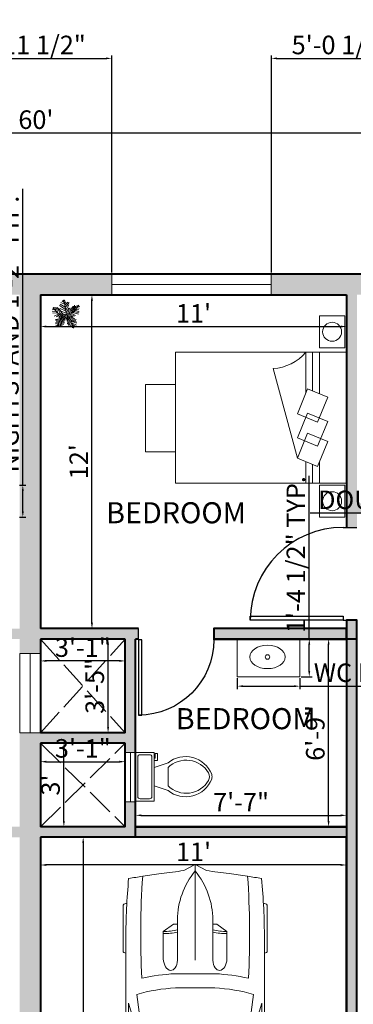
# Model space of a CAD drawing. Units: inches. Extents: x 529 to 1442, y 1029 to 1677.
# Tile 5 of 7: x 991 to 1135, y 1252 to 1677. Entities that reach past the tile are written whole.
import ezdxf

# ---------------------------------------------------------------- set-up
doc = ezdxf.new("R2010")
doc.units = ezdxf.units.IN
doc.linetypes.add('ACAD_ISO02W100', pattern=[15, 12, -3])
for name, color, linetype, lineweight in [('A-ANNO-DIMS', 2, 'Continuous', 18), ('A-AREA-IDEN', 7, 'Continuous', 25), ('A-DOOR', 4, 'Continuous', 25), ('A-EQPM-VEHL', 8, 'Continuous', 13), ('A-FLOR-FIXT', 9, 'Continuous', 18), ('A-FLOR-OVHD', 8, 'ACAD_ISO02W100', 18), ('A-FURN', 8, 'Continuous', 18), ('A-WALL-PATT', 252, 'Continuous', 13), ('tree', 70, 'Continuous', 13), ('wall', 7, 'Continuous', 40), ('window', 52, 'Continuous', 18)]:
    doc.layers.add(name, color=color, linetype=linetype, lineweight=lineweight)
doc.styles.get("Standard").update_dxf_attribs({"font": 'arial.ttf'})
doc.dimstyles.new('ISO-25', dxfattribs={"dimtxt": 8, "dimasz": 2.5, "dimexe": 1.25, "dimexo": 0.625, "dimtad": 1, "dimdec": 0, "dimlunit": 4, "dimtxsty": 'Standard', "dimcen": 2.5, "dimadec": 0, "dimazin": 0, "dimtfac": 1, "dimtdec": 0, "dimtmove": 0, "dimatfit": 3, "dimfxl": 1, "dimarcsym": 0})

# ---------------------------------------------------------------- blocks, each defined once
blk = doc.blocks.new('*U2')
for p, q in [((0, 0), (0, -6)), ((40, 0), (40, -6))]:
    blk.add_line(p, q)
blk.add_lwpolyline([(0, 0), (0, 40), (1.75, 40), (1.75, 0)], close=True)
blk.add_arc((0, 0), 40, 0, 90)
blk = doc.blocks.new('*U4')
for p, q in [((9.5, -6), (9.5, -2)), ((-8, -8.5), (-8, -8)), ((-7, -8), (-7, -9.5)), ((-4, -8), (-6, -14)), ((4, -8), (6, -14)), ((-10, -8.5), (-8, -8.5)), ((-10, -9.5), (-10, -8.5)), ((-7, -9.5), (-10, -9.5)), ((4, -14), (-4, -14))]:
    blk.add_line(p, q)
blk.add_lwpolyline([(10.5, -8), (10.5, 0), (-10.5, 0), (-10.5, -8)], close=True)
for points in [[(-9.5, -2), (-9.5, -6)], [(8.5, -1), (-8.5, -1)], [(-8.5, -7), (8.5, -7)]]:
    blk.add_lwpolyline(points)
for centre, radius, start, end in [((-8.62, -1.88), 0.884, 81.8699, 188.1301), ((8.62, -1.88), 0.884, 351.8699, 98.1301), ((-8.62, -6.12), 0.884, 171.8699, 278.1301), ((8.62, -6.12), 0.884, 261.8699, 8.1301), ((3.52, -21.58), 12.17, 141.4691, 247.9714), ((4.2, -21.82), 11.33, 136.3677, 238.9468), ((-3.52, -21.58), 12.17, 292.0284, 38.5307), ((-4.2, -21.82), 11.33, 301.053, 43.6321), ((0, -27.88), 4, 245.7318, 294.2682), ((0, -29), 4, 254.8605, 285.1395)]:
    blk.add_arc(centre, radius, start, end)
blk = doc.blocks.new('*U6')
for p, q in [((21.1, 37.41), (21.1, 36.83)), ((46.55, 38.89), (22.35, 38.89)), ((47.8, 37.39), (47.8, 37.41)), ((135.45, 37.07), (135.45, 37.41)), ((136.7, 38.89), (160.9, 38.89)), ((162.15, 37.41), (162.15, 36.77)), ((87.99, 31.87), (74.76, 35.92)), ((134.31, 35.6), (119.29, 31.78)), ((186.47, -33.5), (186.47, 33.5)), ((188.4, -32.76), (188.4, 32.76)), ((70.03, 31.54), (86.41, 29.35)), ((138.42, 29.35), (157.25, 29.35)), ((186.47, 29.35), (167.01, 29.35)), ((164.52, 26.39), (164.52, -26.39)), ((32.27, 11.63), (36.13, 17.17)), ((36.13, 17.17), (50.94, 17.17)), ((32.12, 9.51), (32.12, 11.15)), ((58.92, -10.77), (58.92, 10.77)), ((3.27, 6.13), (0.1, 0.41)), ((29.77, 9.51), (51.68, 9.51)), ((66.55, -10.53), (66.55, 10.53)), ((82.74, 8.5), (82.74, -8.5)), ((186.47, -10.53), (186.47, 10.53)), ((0, 0), (51.68, 0)), ((0.1, -0.41), (3.27, -6.13)), ((29.77, -9.51), (51.68, -9.51)), ((32.12, -9.51), (32.12, -11.15)), ((32.27, -11.63), (36.13, -17.17)), ((36.13, -17.17), (50.94, -17.17)), ((86.41, -29.35), (70.03, -31.54)), ((134.31, -35.6), (119.29, -31.78)), ((157.25, -29.35), (138.42, -29.35)), ((167.01, -29.35), (186.47, -29.35)), ((21.1, -37.41), (21.1, -36.83)), ((87.99, -31.87), (74.76, -35.92)), ((135.45, -37.07), (135.45, -37.41)), ((162.15, -37.41), (162.15, -36.77)), ((46.55, -38.89), (22.35, -38.89)), ((47.8, -37.39), (47.8, -37.41)), ((136.7, -38.89), (160.9, -38.89))]:
    blk.add_line(p, q)
for centre, major_axis, ratio, start_param, end_param in [((41.19, -490.86), (0, 528.23), 0.842304, 0.00281, 0.075598), ((22.35, 37.41), (0, -1.48), 0.842304, 3.141593, 4.712389), ((64.48, -10555.62), (0, 10593.03), 0.842304, -0.013397, 0.002797), ((46.55, 37.41), (0, 1.48), 0.842304, -1.570796, 0), ((136.7, 37.41), (0, -1.48), 0.842304, 3.141593, 4.712389), ((160.9, 37.41), (0, 1.48), 0.842304, -1.570796, 0), ((180.63, 35.84), (0, 2.22), 0.842304, -0.013017, 1.249894), ((64.48, -10556.36), (0, 10595.31), 0.842304, -0.013397, -0.013017), ((183.98, 32.76), (0, -5.25), 0.842304, 1.570796, 3.128196), ((266.03, -27.52), (0, 313.31), 0.842304, 1.367076, 1.39176), ((64.48, -10555.62), (0, -10591.55), 0.842304, 3.133765, 3.140441), ((95.79, -3666.35), (0, -3698.24), 0.842304, 3.134049, 3.144098), ((183.98, 33.5), (0, -2.96), 0.842304, 1.570796, 3.128196), ((259.18, -27.52), (0, -305.3), 0.842304, 4.528606, 4.561838), ((37.47, -593.96), (0, -623.33), 0.842304, 3.096046, 3.200911), ((134.4, 5.39), (0, -89.78), 0.842304, 4.449482, 4.652344), ((135.29, 5.39), (0, 81.77), 0.842304, 1.245306, 1.50788), ((149.6, 2.8), (0, -79.58), 0.842304, 4.372215, 4.640744), ((17.08, 0), (0, 147.02), 0.842304, 4.511394, 4.913384), ((35.91, 0), (0, 147.02), 0.842304, 4.511394, 4.913384), ((167.01, 26.39), (0, 2.96), 0.842304, 0, 1.570796), ((-204.49, 52.4), (0, -250.96), 0.842304, 1.385369, 1.434372), ((13.04, 17.01), (0, 27.42), 0.842304, 4.435146, 4.718221), ((14.2, 17.01), (0, 27.42), 0.842304, 4.435146, 4.718221), ((50.79, 13.34), (6.34, -0.36), 0.603834, -1.395552, 1.581315), ((32.75, 11.15), (0, 0.74), 0.842304, 0.879714, 1.570796), ((29.77, -46.66), (0, 56.17), 0.842304, 0, 0.590319), ((0.62, 0), (0, -0.74), 0.842304, 4.131459, 5.293319), ((29.77, 46.66), (0, 56.17), 0.842304, 2.551274, 3.141593), ((-204.49, -52.4), (0, 250.96), 0.842304, -1.434372, -1.385369), ((13.04, -17.01), (0, -27.42), 0.842304, 1.564964, 1.848039), ((14.2, -17.01), (0, -27.42), 0.842304, 1.564964, 1.848039), ((135.29, -5.39), (0, -81.77), 0.842304, -1.50788, -1.245306), ((149.6, -2.8), (0, -79.58), 0.842304, -1.499151, -1.230623), ((32.75, -11.15), (0, -0.74), 0.842304, 4.712389, 5.403472), ((134.4, -5.39), (0, -89.78), 0.842304, -1.510751, -1.307889), ((259.18, 27.52), (0, 305.3), 0.842304, 1.721348, 1.754579), ((167.01, -26.39), (0, -2.96), 0.842304, 4.712389, 6.283185), ((266.03, 27.52), (0, 313.31), 0.842304, 1.749832, 1.774517), ((37.47, 593.96), (0, -623.33), 0.842304, -0.059319, 0.045547), ((95.79, 3666.35), (0, -3698.24), 0.842304, -0.002505, 0.007544), ((41.19, 490.86), (0, -528.23), 0.842304, -0.075598, -0.00281), ((64.48, 10555.62), (0, 10593.03), 0.842304, 3.138796, 3.15499), ((64.48, 10555.62), (0, -10591.55), 0.842304, 0.001152, 0.007828), ((180.63, -35.84), (0, -2.22), 0.842304, -1.249894, 0.013017), ((183.98, -33.5), (0, 2.96), 0.842304, 3.15499, 4.712389), ((183.98, -32.76), (0, -5.25), 0.842304, 0.013397, 1.570796), ((22.35, -37.41), (0, 1.48), 0.842304, 1.570796, 3.141593), ((46.55, -37.41), (0, -1.48), 0.842304, 0, 1.570796), ((136.7, -37.41), (0, -1.48), 0.842304, -1.570796, 0), ((160.9, -37.41), (0, 1.48), 0.842304, 3.141593, 4.712389), ((64.48, 10556.36), (0, 10595.31), 0.842304, 3.15461, 3.15499)]:
    blk.add_ellipse(centre, major_axis=major_axis, ratio=ratio, start_param=start_param, end_param=end_param)
at = {"extrusion": (0, 0, -1)}
blk.add_ellipse((50.79, -13.34), major_axis=(6.34, 0.36), ratio=0.603834, start_param=-1.395552, end_param=1.581315, dxfattribs=at)
blk = doc.blocks.new('*U12')
for p, q in [((-5.114, 28.097), (-24.676, 40.636)), ((-7.288, 39.707), (-21.778, 46.673)), ((-8.737, 47.138), (-17.069, 52.711)), ((-10.186, 53.64), (-13.084, 55.962)), ((0, 0), (-10.5, 57)), ((-9.099, 51.782), (-6.563, 55.962)), ((-7.65, 43.423), (-2.578, 49.46)), ((-5.839, 35.992), (4.667, 48.067)), ((-5.114, 27.632), (10.463, 46.673)), ((-47.498, 19.737), (-55.83, 18.344)), ((-40.615, 13.7), (-55.105, 10.913)), ((-31.5, 4.5), (-52.5, 25.5)), ((-33.37, 6.269), (-52.207, 5.34)), ((-48.585, 21.131), (-49.309, 29.026)), ((-28.299, 3.483), (-47.86, -5.805)), ((-43.513, 28.561), (-42.427, 15.558)), ((-38.442, 26.239), (-34.819, 7.663)), ((-21.416, 3.018), (-38.079, -8.128)), ((-35.544, 28.097), (-24.314, 3.947)), ((0, 0), (-31.5, 4.5)), ((-14.533, 2.09), (-30.834, 25.31)), ((-15.982, 2.09), (-30.11, -9.521)), ((-3.665, 19.273), (-27.574, 35.527)), ((-24.314, 23.917), (-2.941, 13.7)), ((0, 0), (-22.5, -19.5)), ((-6.563, 1.161), (-21.416, -8.128)), ((-20.691, 13.7), (-1.129, 4.876)), ((-2.941, 16.486), (8.652, 37.85)), ((-1.129, 6.734), (9.014, 26.704)), ((0, 0), (27, 9)), ((0, 0), (18, -22.5)), ((3.942, 1.625), (11.187, 24.381)), ((6.478, 1.625), (26.04, -8.592)), ((10.101, 3.483), (17.708, 26.239)), ((11.187, 3.483), (30.749, -5.805)), ((16.259, 5.805), (23.142, 31.348)), ((18.07, 5.805), (35.096, -3.483)), ((22.055, 7.198), (27.489, 32.277)), ((24.229, 7.663), (46.688, 1.625)), ((27, 9), (48, 36)), ((27.127, 9.056), (31.112, 35.992)), ((29.662, 12.307), (48.137, 6.269)), ((31.836, 30.883), (32.561, 16.486)), ((33.285, 16.486), (48.862, 10.913)), ((35.096, 32.741), (37.27, 22.524)), ((36.183, 19.737), (48.137, 17.88)), ((38.719, 34.134), (41.979, 28.561)), ((40.53, 25.775), (48.862, 24.846)), ((43.791, 29.954), (51.036, 30.883)), ((44.153, 36.456), (45.239, 32.741)), ((-17.431, -15.094), (-42.789, -18.809)), ((-28.299, -29.026), (-42.789, -31.348)), ((-24.314, -21.596), (-42.427, -22.06)), ((-30.834, -34.135), (-42.427, -35.528)), ((-26.849, -26.24), (-40.253, -25.775)), ((-22.5, -19.5), (-37.5, -45)), ((-32.646, -36.921), (-31.921, -44.352)), ((-15.257, -12.772), (-30.11, -12.772)), ((-29.023, -30.884), (-27.936, -43.887)), ((-25.038, -23.918), (-22.865, -45.281)), ((-20.691, -18.345), (-17.793, -44.352)), ((-6.563, -5.805), (-19.967, -9.985)), ((-17.069, -15.094), (-12.721, -40.172)), ((-13.446, -11.378), (-8.737, -32.741)), ((-9.461, -8.592), (-6.201, -23.453)), ((-4.752, -3.483), (-3.665, -14.629)), ((2.493, -3.019), (-1.491, -20.202)), ((1.769, -2.555), (24.229, -9.521)), ((5.029, -6.27), (2.131, -25.775)), ((9.014, -11.378), (3.58, -35.992)), ((14.085, -16.951), (6.478, -40.172)), ((7.565, -9.056), (32.198, -14.629)), ((18.07, -22.524), (8.289, -45.745)), ((12.274, -15.094), (36.907, -18.809)), ((20.244, -30.419), (15.897, -44.816)), ((16.259, -19.738), (36.183, -22.989)), ((18, -22.5), (27, -52.5)), ((18.433, -22.524), (40.53, -29.026)), ((19.157, -25.311), (38.719, -33.206)), ((22.78, -37.85), (19.519, -48.532)), ((21.331, -32.741), (39.081, -40.636)), ((-34.457, -39.708), (-40.978, -42.494)), ((22.78, -38.314), (34.372, -44.816)), ((24.591, -45.745), (23.142, -50.854)), ((24.591, -43.423), (30.749, -47.603)), ((26.764, -49.925), (28.213, -50.854))]:
    blk.add_line(p, q)
blk = doc.blocks.new('*D19')
at = {"layer": 'A-ANNO-DIMS', "color": 0, "lineweight": -2, "transparency": 16777216}
for p, q in [((1000.38, 1557.19), (1000.38, 1542.87)), ((1132.38, 1557.19), (1132.38, 1542.87)), ((1002.88, 1544.12), (1129.88, 1544.12))]:
    blk.add_line(p, q, dxfattribs=at)
at = {"layer": 'A-ANNO-DIMS', "color": 0, "lineweight": 100, "transparency": 16777216}
for points in [[(1002.88, 1544.54), (1002.88, 1543.71), (1000.38, 1544.12)], [(1129.88, 1544.54), (1129.88, 1543.71), (1132.38, 1544.12)]]:
    blk.add_solid(points, dxfattribs=at)
at = {"layer": 'Defpoints', "color": 0, "lineweight": 100, "transparency": 16777216}
for p in [(1000.38, 1557.81), (1132.38, 1557.81), (1132.38, 1544.12)]:
    blk.add_point(p, dxfattribs=at)
at = {"layer": 'A-ANNO-DIMS', "color": 0, "transparency": 16777216, "insert": (1066.38, 1548.76), "char_height": 8, "attachment_point": 5}
blk.add_mtext("11'", dxfattribs=at)
blk = doc.blocks.new('*D20')
at = {"layer": 'A-ANNO-DIMS', "color": 0, "lineweight": -2, "transparency": 16777216}
for p, q in [((1001.01, 1557.81), (1023.8, 1557.81)), ((1022.55, 1416.31), (1022.55, 1555.31)), ((1001.01, 1413.81), (1023.8, 1413.81))]:
    blk.add_line(p, q, dxfattribs=at)
at = {"layer": 'A-ANNO-DIMS', "color": 0, "lineweight": 100, "transparency": 16777216}
for points in [[(1022.14, 1555.31), (1022.97, 1555.31), (1022.55, 1557.81)], [(1022.14, 1416.31), (1022.97, 1416.31), (1022.55, 1413.81)]]:
    blk.add_solid(points, dxfattribs=at)
at = {"layer": 'Defpoints', "color": 0, "lineweight": 100, "transparency": 16777216}
for p in [(1000.38, 1557.81), (1022.55, 1557.81), (1000.38, 1413.81)]:
    blk.add_point(p, dxfattribs=at)
at = {"layer": 'A-ANNO-DIMS', "color": 0, "transparency": 16777216, "insert": (1017.91, 1485.81), "char_height": 8, "attachment_point": 5, "rotation": 90}
blk.add_mtext("12'", dxfattribs=at)
blk = doc.blocks.new('*D33')
at = {"layer": 'A-ANNO-DIMS', "color": 0, "lineweight": -2, "transparency": 16777216}
for p, q in [((1000.38, 1323.19), (1000.38, 1310.57)), ((1132.38, 1323.19), (1132.38, 1310.57)), ((1129.88, 1311.82), (1002.88, 1311.82))]:
    blk.add_line(p, q, dxfattribs=at)
at = {"layer": 'A-ANNO-DIMS', "color": 0, "lineweight": 100, "transparency": 16777216}
for points in [[(1002.88, 1312.24), (1002.88, 1311.41), (1000.38, 1311.82)], [(1129.88, 1312.24), (1129.88, 1311.41), (1132.38, 1311.82)]]:
    blk.add_solid(points, dxfattribs=at)
at = {"layer": 'Defpoints', "color": 0, "lineweight": 100, "transparency": 16777216}
for p in [(1000.38, 1323.81), (1132.38, 1323.81), (1000.38, 1311.82)]:
    blk.add_point(p, dxfattribs=at)
at = {"layer": 'A-ANNO-DIMS', "color": 0, "transparency": 16777216, "insert": (1066.38, 1316.46), "char_height": 8, "attachment_point": 5}
blk.add_mtext("11'", dxfattribs=at)
blk = doc.blocks.new('*D34')
at = {"layer": 'A-ANNO-DIMS', "color": 0, "lineweight": -2, "transparency": 16777216}
for p, q in [((1001.01, 1323.81), (1020.03, 1323.81)), ((1018.78, 1321.31), (1018.78, 1158.31)), ((1001.01, 1155.81), (1020.03, 1155.81))]:
    blk.add_line(p, q, dxfattribs=at)
at = {"layer": 'A-ANNO-DIMS', "color": 0, "lineweight": 100, "transparency": 16777216}
for points in [[(1018.36, 1321.31), (1019.19, 1321.31), (1018.78, 1323.81)], [(1018.36, 1158.31), (1019.19, 1158.31), (1018.78, 1155.81)]]:
    blk.add_solid(points, dxfattribs=at)
at = {"layer": 'Defpoints', "color": 0, "lineweight": 100, "transparency": 16777216}
for p in [(1000.38, 1323.81), (1000.38, 1155.81), (1018.78, 1155.81)]:
    blk.add_point(p, dxfattribs=at)
at = {"layer": 'A-ANNO-DIMS', "color": 0, "transparency": 16777216, "insert": (1014.13, 1239.81), "char_height": 8, "attachment_point": 5, "rotation": 90}
blk.add_mtext("14'", dxfattribs=at)
blk = doc.blocks.new('*D49')
at = {"layer": 'A-ANNO-DIMS', "color": 0, "lineweight": -2, "transparency": 16777216}
for p, q in [((1036.26, 1409.31), (1028.27, 1409.31)), ((1029.52, 1371.31), (1029.52, 1406.81)), ((1036.26, 1368.81), (1028.27, 1368.81))]:
    blk.add_line(p, q, dxfattribs=at)
at = {"layer": 'A-ANNO-DIMS', "color": 0, "lineweight": 100, "transparency": 16777216}
for points in [[(1029.1, 1406.81), (1029.93, 1406.81), (1029.52, 1409.31)], [(1029.1, 1371.31), (1029.93, 1371.31), (1029.52, 1368.81)]]:
    blk.add_solid(points, dxfattribs=at)
at = {"layer": 'Defpoints', "color": 0, "lineweight": 100, "transparency": 16777216}
for p in [(1029.52, 1409.31), (1036.88, 1409.31), (1036.88, 1368.81)]:
    blk.add_point(p, dxfattribs=at)
at = {"layer": 'A-ANNO-DIMS', "color": 0, "transparency": 16777216, "insert": (1024.81, 1389.06), "char_height": 8, "attachment_point": 5, "rotation": 90}
blk.add_mtext('3\'-5"', dxfattribs=at)
blk = doc.blocks.new('*D50')
at = {"layer": 'A-ANNO-DIMS', "color": 0, "lineweight": -2, "transparency": 16777216}
for p, q in [((1000.38, 1408.69), (1000.38, 1398.62)), ((1036.88, 1408.69), (1036.88, 1398.62)), ((1034.38, 1399.87), (1002.88, 1399.87))]:
    blk.add_line(p, q, dxfattribs=at)
at = {"layer": 'A-ANNO-DIMS', "color": 0, "lineweight": 100, "transparency": 16777216}
for points in [[(1002.88, 1400.28), (1002.88, 1399.45), (1000.38, 1399.87)], [(1034.38, 1400.28), (1034.38, 1399.45), (1036.88, 1399.87)]]:
    blk.add_solid(points, dxfattribs=at)
at = {"layer": 'Defpoints', "color": 0, "lineweight": 100, "transparency": 16777216}
for p in [(1000.38, 1409.31), (1036.88, 1409.31), (1000.38, 1399.87)]:
    blk.add_point(p, dxfattribs=at)
at = {"layer": 'A-ANNO-DIMS', "color": 0, "transparency": 16777216, "insert": (1018.63, 1404.58), "char_height": 8, "attachment_point": 5}
blk.add_mtext('3\'-1"', dxfattribs=at)
blk = doc.blocks.new('*D51')
at = {"layer": 'A-ANNO-DIMS', "color": 0, "lineweight": -2, "transparency": 16777216}
for p, q in [((1000.38, 1363.69), (1000.38, 1355.13)), ((1036.88, 1363.69), (1036.88, 1355.13)), ((1002.88, 1356.38), (1034.38, 1356.38))]:
    blk.add_line(p, q, dxfattribs=at)
at = {"layer": 'A-ANNO-DIMS', "color": 0, "lineweight": 100, "transparency": 16777216}
for points in [[(1002.88, 1356.8), (1002.88, 1355.97), (1000.38, 1356.38)], [(1034.38, 1356.8), (1034.38, 1355.97), (1036.88, 1356.38)]]:
    blk.add_solid(points, dxfattribs=at)
at = {"layer": 'Defpoints', "color": 0, "lineweight": 100, "transparency": 16777216}
for p in [(1000.38, 1364.31), (1036.88, 1364.31), (1036.88, 1356.38)]:
    blk.add_point(p, dxfattribs=at)
at = {"layer": 'A-ANNO-DIMS', "color": 0, "transparency": 16777216, "insert": (1018.63, 1361.1), "char_height": 8, "attachment_point": 5}
blk.add_mtext('3\'-1"', dxfattribs=at)
blk = doc.blocks.new('*D52')
at = {"layer": 'A-ANNO-DIMS', "color": 0, "lineweight": -2, "transparency": 16777216}
for p, q in [((1001.01, 1364.31), (1011.69, 1364.31)), ((1010.44, 1330.81), (1010.44, 1361.81)), ((1001.01, 1328.31), (1011.69, 1328.31))]:
    blk.add_line(p, q, dxfattribs=at)
at = {"layer": 'A-ANNO-DIMS', "color": 0, "lineweight": 100, "transparency": 16777216}
for points in [[(1010.02, 1361.81), (1010.85, 1361.81), (1010.44, 1364.31)], [(1010.02, 1330.81), (1010.85, 1330.81), (1010.44, 1328.31)]]:
    blk.add_solid(points, dxfattribs=at)
at = {"layer": 'Defpoints', "color": 0, "lineweight": 100, "transparency": 16777216}
for p in [(1000.38, 1364.31), (1010.44, 1364.31), (1000.38, 1328.31)]:
    blk.add_point(p, dxfattribs=at)
at = {"layer": 'A-ANNO-DIMS', "color": 0, "transparency": 16777216, "insert": (1005.72, 1346.31), "char_height": 8, "attachment_point": 5, "rotation": 90}
blk.add_mtext("3'", dxfattribs=at)
blk = doc.blocks.new('*D53')
at = {"layer": 'A-ANNO-DIMS', "color": 0, "lineweight": -2, "transparency": 16777216}
for p, q in [((1131.76, 1409.31), (1123.4, 1409.31)), ((1124.65, 1330.81), (1124.65, 1406.81)), ((1131.76, 1328.31), (1123.4, 1328.31))]:
    blk.add_line(p, q, dxfattribs=at)
at = {"layer": 'A-ANNO-DIMS', "color": 0, "lineweight": 100, "transparency": 16777216}
for points in [[(1124.23, 1406.81), (1125.06, 1406.81), (1124.65, 1409.31)], [(1124.23, 1330.81), (1125.06, 1330.81), (1124.65, 1328.31)]]:
    blk.add_solid(points, dxfattribs=at)
at = {"layer": 'Defpoints', "color": 0, "lineweight": 100, "transparency": 16777216}
for p in [(1124.65, 1409.31), (1132.38, 1409.31), (1132.38, 1328.31)]:
    blk.add_point(p, dxfattribs=at)
at = {"layer": 'A-ANNO-DIMS', "color": 0, "transparency": 16777216, "insert": (1119.94, 1368.81), "char_height": 8, "attachment_point": 5, "rotation": 90}
blk.add_mtext('6\'-9"', dxfattribs=at)
blk = doc.blocks.new('*D54')
at = {"layer": 'A-ANNO-DIMS', "color": 0, "lineweight": -2, "transparency": 16777216}
for p, q in [((1041.38, 1328.94), (1041.38, 1334.49)), ((1132.38, 1328.94), (1132.38, 1334.49)), ((1043.88, 1333.24), (1129.88, 1333.24))]:
    blk.add_line(p, q, dxfattribs=at)
at = {"layer": 'A-ANNO-DIMS', "color": 0, "lineweight": 100, "transparency": 16777216}
for points in [[(1043.88, 1333.66), (1043.88, 1332.83), (1041.38, 1333.24)], [(1129.88, 1333.66), (1129.88, 1332.83), (1132.38, 1333.24)]]:
    blk.add_solid(points, dxfattribs=at)
at = {"layer": 'Defpoints', "color": 0, "lineweight": 100, "transparency": 16777216}
for p in [(1132.38, 1333.24), (1041.38, 1328.31), (1132.38, 1328.31)]:
    blk.add_point(p, dxfattribs=at)
at = {"layer": 'A-ANNO-DIMS', "color": 0, "transparency": 16777216, "insert": (1086.88, 1337.87), "char_height": 8, "attachment_point": 5}
blk.add_mtext('7\'-7"', dxfattribs=at)
blk = doc.blocks.new('*D55')
at = {"layer": 'A-ANNO-DIMS', "color": 0, "lineweight": -2, "transparency": 16777216}
for p, q in [((638.38, 1567.44), (638.38, 1628.88)), ((640.88, 1627.63), (1355.88, 1627.63)), ((1358.38, 1567.44), (1358.38, 1628.88))]:
    blk.add_line(p, q, dxfattribs=at)
at = {"layer": 'A-ANNO-DIMS', "color": 0, "lineweight": 100, "transparency": 16777216}
for points in [[(640.88, 1628.05), (640.88, 1627.22), (638.38, 1627.63)], [(1355.88, 1628.05), (1355.88, 1627.22), (1358.38, 1627.63)]]:
    blk.add_solid(points, dxfattribs=at)
at = {"layer": 'Defpoints', "color": 0, "lineweight": 100, "transparency": 16777216}
for p in [(1358.38, 1627.63), (638.38, 1566.81), (1358.38, 1566.81)]:
    blk.add_point(p, dxfattribs=at)
at = {"layer": 'A-ANNO-DIMS', "color": 0, "transparency": 16777216, "insert": (998.38, 1632.34), "char_height": 8, "attachment_point": 5}
blk.add_mtext("60'", dxfattribs=at)
blk = doc.blocks.new('WIN-LARGE-PLAN')
blk.add_line((0, 4.5), (68.85, 4.5))
blk.add_lwpolyline([(0, 9), (68.85, 9), (68.85, 0), (0, 0)], close=True)
blk = doc.blocks.new('BED-DOUBLE')
for p, q in [((10.82, 21.21), (49.46, 31.61)), ((0, 17.58), (9.33, 17.58)), ((0, 17.58), (9.33, 17.58)), ((28.37, 17.58), (28.47, 17.58)), ((28.37, 17.58), (28.47, 17.58)), ((38.76, 17.58), (56.44, 17.58)), ((38.76, 17.58), (56.44, 17.58)), ((0, 14.65), (8.12, 14.65)), ((39.74, 14.65), (56.44, 14.65)), ((0, 11.71), (9.09, 11.71)), ((28.13, 11.71), (28.23, 11.71)), ((38.53, 11.71), (56.44, 11.71))]:
    blk.add_line(p, q)
for points in [[(13.54, 73.79), (42.58, 73.79), (42.58, 86.74), (13.54, 86.74)], [(0, 0), (56.44, 0), (56.44, 73.79), (0, 73.79)], [(10.82, 21.21), (21.49, 16.82), (17.9, 8.09), (7.23, 12.48)], [(19.56, 21.21), (30.23, 16.82), (26.64, 8.09), (15.97, 12.48)], [(29.96, 21.21), (40.63, 16.82), (37.04, 8.09), (26.37, 12.48)]]:
    blk.add_lwpolyline(points, close=True)
blk.add_arc((69.23, 32.7), 19.8, 183.1428, 229.758)
blk = doc.blocks.new('NIGHTSTAND')
blk.add_lwpolyline([(0, 0), (13.77, 0), (13.77, 10.99), (0, 10.99)], close=True)
blk.add_circle((6.88, 5.5), 4.1)
blk = doc.blocks.new('WASHBASIN')
blk.add_lwpolyline([(0, 16.29), (27.02, 16.29), (27.02, 0), (0, 0)], close=True)
blk.add_circle((13.05, 8.54), 0.991)
blk.add_ellipse((13.05, 8.54), major_axis=(7.63, 0), ratio=0.659433)
blk = doc.blocks.new('*D77')
at = {"layer": 'A-ANNO-DIMS', "color": 0, "lineweight": -2, "transparency": 16777216}
for p, q in [((1262.64, 1475.94), (1262.64, 1462.3)), ((1349.38, 1475.94), (1349.38, 1462.3)), ((1262.64, 1463.55), (1116.74, 1463.55)), ((1346.88, 1463.55), (1265.14, 1463.55))]:
    blk.add_line(p, q, dxfattribs=at)
at = {"layer": 'A-ANNO-DIMS', "color": 0, "lineweight": 100, "transparency": 16777216}
for points in [[(1265.14, 1463.97), (1265.14, 1463.13), (1262.64, 1463.55)], [(1346.88, 1463.97), (1346.88, 1463.13), (1349.38, 1463.55)]]:
    blk.add_solid(points, dxfattribs=at)
at = {"layer": 'Defpoints', "color": 0, "lineweight": 100, "transparency": 16777216}
for p in [(1262.64, 1476.56), (1349.38, 1476.56), (1262.64, 1463.55)]:
    blk.add_point(p, dxfattribs=at)
at = {"layer": 'A-ANNO-DIMS', "color": 0, "transparency": 16777216, "insert": (1188.44, 1468.32), "char_height": 8, "attachment_point": 5}
blk.add_mtext('DOUBLE BED 7\'-2 1/2" TYP.', dxfattribs=at)
blk = doc.blocks.new('*D79')
at = {"layer": 'A-ANNO-DIMS', "color": 0, "lineweight": -2, "transparency": 16777216}
for p, q in [((992.73, 1475.66), (992.73, 1603.54)), ((991.29, 1475.66), (993.98, 1475.66)), ((992.73, 1464.39), (992.73, 1473.16)), ((991.29, 1461.89), (993.98, 1461.89))]:
    blk.add_line(p, q, dxfattribs=at)
at = {"layer": 'A-ANNO-DIMS', "color": 0, "lineweight": 100, "transparency": 16777216}
for points in [[(992.31, 1473.16), (993.15, 1473.16), (992.73, 1475.66)], [(992.31, 1464.39), (993.15, 1464.39), (992.73, 1461.89)]]:
    blk.add_solid(points, dxfattribs=at)
at = {"layer": 'Defpoints', "color": 0, "lineweight": 100, "transparency": 16777216}
for p in [(990.66, 1475.66), (992.73, 1475.66), (990.66, 1461.89)]:
    blk.add_point(p, dxfattribs=at)
at = {"layer": 'A-ANNO-DIMS', "color": 0, "transparency": 16777216, "insert": (987.97, 1540.85), "char_height": 8, "attachment_point": 5, "rotation": 90}
blk.add_mtext('NIGHTSTAND 1\'-2" TYP.', dxfattribs=at)
blk = doc.blocks.new('*D85')
at = {"layer": 'A-ANNO-DIMS', "color": 0, "lineweight": -2, "transparency": 16777216}
for p, q in [((1085.24, 1392.4), (1085.24, 1387.72)), ((1112.26, 1392.4), (1112.26, 1387.72)), ((1087.74, 1388.97), (1109.76, 1388.97)), ((1112.26, 1388.97), (1223.47, 1388.97))]:
    blk.add_line(p, q, dxfattribs=at)
at = {"layer": 'A-ANNO-DIMS', "color": 0, "lineweight": 100, "transparency": 16777216}
for points in [[(1087.74, 1389.38), (1087.74, 1388.55), (1085.24, 1388.97)], [(1109.76, 1389.38), (1109.76, 1388.55), (1112.26, 1388.97)]]:
    blk.add_solid(points, dxfattribs=at)
at = {"layer": 'Defpoints', "color": 0, "lineweight": 100, "transparency": 16777216}
for p in [(1085.24, 1393.02), (1112.26, 1393.02), (1112.26, 1388.97)]:
    blk.add_point(p, dxfattribs=at)
at = {"layer": 'A-ANNO-DIMS', "color": 0, "transparency": 16777216, "insert": (1169.11, 1393.73), "char_height": 8, "attachment_point": 5}
blk.add_mtext('WC BASIN 2\'-3" TYP.', dxfattribs=at)
blk = doc.blocks.new('*D86')
at = {"layer": 'A-ANNO-DIMS', "color": 0, "lineweight": -2, "transparency": 16777216}
for p, q in [((1116.31, 1409.31), (1116.31, 1479.71)), ((1112.88, 1409.31), (1117.56, 1409.31)), ((1116.31, 1395.52), (1116.31, 1406.81)), ((1112.88, 1393.02), (1117.56, 1393.02))]:
    blk.add_line(p, q, dxfattribs=at)
at = {"layer": 'A-ANNO-DIMS', "color": 0, "lineweight": 100, "transparency": 16777216}
for points in [[(1115.89, 1406.81), (1116.73, 1406.81), (1116.31, 1409.31)], [(1115.89, 1395.52), (1116.73, 1395.52), (1116.31, 1393.02)]]:
    blk.add_solid(points, dxfattribs=at)
at = {"layer": 'Defpoints', "color": 0, "lineweight": 100, "transparency": 16777216}
for p in [(1112.26, 1409.31), (1116.31, 1409.31), (1112.26, 1393.02)]:
    blk.add_point(p, dxfattribs=at)
at = {"layer": 'A-ANNO-DIMS', "color": 0, "transparency": 16777216, "insert": (1111.55, 1445.76), "char_height": 8, "attachment_point": 5, "rotation": 90}
blk.add_mtext('1\'-4 1/2" TYP.', dxfattribs=at)
blk = doc.blocks.new('*D102')
at = {"layer": 'A-ANNO-DIMS', "color": 0, "lineweight": -2, "transparency": 16777216}
for p, q in [((959.72, 1567.44), (959.72, 1661.06)), ((1031.09, 1567.44), (1031.09, 1661.06)), ((962.22, 1659.81), (1028.59, 1659.81))]:
    blk.add_line(p, q, dxfattribs=at)
at = {"layer": 'A-ANNO-DIMS', "color": 0, "lineweight": 100, "transparency": 16777216}
for points in [[(962.22, 1660.23), (962.22, 1659.4), (959.72, 1659.81)], [(1028.59, 1660.23), (1028.59, 1659.4), (1031.09, 1659.81)]]:
    blk.add_solid(points, dxfattribs=at)
at = {"layer": 'Defpoints', "color": 0, "lineweight": 100, "transparency": 16777216}
for p in [(1031.09, 1659.81), (959.72, 1566.81), (1031.09, 1566.81)]:
    blk.add_point(p, dxfattribs=at)
at = {"layer": 'A-ANNO-DIMS', "color": 0, "transparency": 16777216, "insert": (995.41, 1664.57), "char_height": 8, "attachment_point": 5}
blk.add_mtext('5\'-11 1/2"', dxfattribs=at)
blk = doc.blocks.new('*D103')
at = {"layer": 'A-ANNO-DIMS', "color": 0, "lineweight": -2, "transparency": 16777216}
for p, q in [((1099.95, 1567.44), (1099.95, 1661.06)), ((1160.38, 1567.44), (1160.38, 1661.06)), ((1102.45, 1659.81), (1157.88, 1659.81))]:
    blk.add_line(p, q, dxfattribs=at)
at = {"layer": 'A-ANNO-DIMS', "color": 0, "lineweight": 100, "transparency": 16777216}
for points in [[(1102.45, 1660.23), (1102.45, 1659.4), (1099.95, 1659.81)], [(1157.88, 1660.23), (1157.88, 1659.4), (1160.38, 1659.81)]]:
    blk.add_solid(points, dxfattribs=at)
at = {"layer": 'Defpoints', "color": 0, "lineweight": 100, "transparency": 16777216}
for p in [(1160.38, 1659.81), (1099.95, 1566.81), (1160.38, 1566.81)]:
    blk.add_point(p, dxfattribs=at)
at = {"layer": 'A-ANNO-DIMS', "color": 0, "transparency": 16777216, "insert": (1130.17, 1664.57), "char_height": 8, "attachment_point": 5}
blk.add_mtext('5\'-0 1/2"', dxfattribs=at)

msp = doc.modelspace()

# ---------------------------------------------------------------- hatches: boundary and pattern name
at = {"layer": 'A-WALL-PATT'}
h = msp.add_hatch(color=256, dxfattribs=at)
h.dxf.hatch_style = 1
h.paths.add_polyline_path([(1031.09, 1566.81), (959.72, 1566.81), (959.72, 1557.81), (991.38, 1557.81), (1031.09, 1557.81)])
h.paths.add_polyline_path([(1000.38, 1557.81), (991.38, 1557.81), (991.38, 1413.81), (991.38, 1409.31), (1000.38, 1409.31)])
h.paths.add_polyline_path([(991.38, 1413.81), (904.07, 1413.81), (904.07, 1409.31), (991.38, 1409.31)])
h.paths.add_polyline_path([(931.38, 1409.31), (926.88, 1409.31), (926.88, 1359.54), (931.38, 1359.54)])
h.paths.add_polyline_path([(854.88, 1257.31), (835.24, 1257.31), (835.24, 1252.81), (854.36, 1252.81, -0.003534), (854.88, 1252.81)])
h.paths.add_polyline_path([(859.38, 1323.81), (991.38, 1323.81), (991.38, 1328.31), (931.38, 1328.31), (854.88, 1328.31), (854.88, 1155.81), (859.38, 1155.81)])
h.paths.add_polyline_path([(1000.38, 1323.81), (991.38, 1323.81), (991.38, 1155.81), (991.38, 1146.81), (1000.35, 1146.81), (1000.38, 1155.81)])
h.paths.add_polyline_path([(1041.38, 1328.31), (1000.38, 1328.31), (1000.38, 1323.81), (1041.38, 1323.81)])
h.paths.add_polyline_path([(1041.38, 1339.12), (1036.88, 1339.12), (1036.88, 1328.31), (1041.38, 1328.31)])
h.paths.add_polyline_path([(1000.38, 1328.31), (991.38, 1328.31), (991.38, 1323.81), (1000.38, 1323.81)])
h.paths.add_polyline_path([(1041.38, 1409.31), (1036.88, 1409.31), (1036.88, 1360.41), (1041.38, 1360.41)])
h.paths.add_polyline_path([(1042.64, 1413.81), (1000.38, 1413.81), (1000.38, 1409.31), (1042.64, 1409.31)])
h = msp.add_hatch(color=256, dxfattribs=at)
h.dxf.hatch_style = 1
h.paths.add_polyline_path([(1132.38, 1328.31), (1041.38, 1328.31), (1041.38, 1323.81), (1132.38, 1323.81)])
h.paths.add_polyline_path([(1132.38, 1413.81), (1075.12, 1413.81), (1075.12, 1409.31), (1132.38, 1409.31)])
h.paths.add_polyline_path([(1246.5, 1566.81), (1191.67, 1566.81), (1191.67, 1557.81), (1246.5, 1557.81)])
h.paths.add_polyline_path([(1160.38, 1566.81), (1099.95, 1566.81), (1099.95, 1557.81), (1132.38, 1557.81), (1160.38, 1557.81)])
h = msp.add_hatch(color=256, dxfattribs=at)
h.dxf.hatch_style = 1
h.paths.add_polyline_path([(1160.38, 1566.81), (1099.95, 1566.81), (1099.95, 1557.81), (1132.38, 1557.81), (1160.38, 1557.81)])
h.paths.add_polyline_path([(1136.88, 1557.81), (1132.38, 1557.81), (1132.38, 1457.46), (1136.88, 1457.46)])
h.paths.add_polyline_path([(1171.8, 1467.81), (1136.88, 1467.81), (1136.88, 1463.31), (1171.8, 1463.31)])
h.paths.add_polyline_path([(1212.38, 1557.81), (1207.88, 1557.81), (1207.88, 1467.81), (1207.88, 1409.31), (1218.04, 1409.31), (1218.04, 1413.81), (1212.38, 1413.81), (1212.38, 1463.31)])
h.paths.add_polyline_path([(1136.88, 1409.31), (1132.38, 1409.31), (1132.38, 1146.81), (1136.88, 1146.81)])
h.paths.add_polyline_path([(1136.88, 1417.46), (1132.38, 1417.46), (1132.38, 1409.31), (1136.88, 1409.31)])
h.paths.add_polyline_path([(1132.38, 1413.81), (1075.12, 1413.81), (1075.12, 1409.31), (1132.38, 1409.31)])
h.paths.add_polyline_path([(1132.38, 1328.31), (1041.38, 1328.31), (1041.38, 1323.81), (1132.38, 1323.81)])
h = msp.add_hatch(color=256, dxfattribs=at)
h.dxf.hatch_style = 1
h.paths.add_polyline_path([(1171.8, 1467.81), (1136.88, 1467.81), (1136.88, 1463.31), (1171.8, 1463.31)])
h.paths.add_polyline_path([(1136.88, 1557.81), (1132.38, 1557.81), (1132.38, 1457.46), (1136.88, 1457.46)])
h.paths.add_polyline_path([(1212.38, 1557.81), (1207.88, 1557.81), (1207.88, 1467.81), (1207.88, 1409.31), (1218.04, 1409.31), (1218.04, 1413.81), (1212.38, 1413.81), (1212.38, 1463.31)])
h = msp.add_hatch(color=256, dxfattribs=at)
h.dxf.hatch_style = 1
h.paths.add_polyline_path([(1259.88, 1228.31), (1187.26, 1228.31), (1187.26, 1226.94), (1187.26, 1223.81), (1259.88, 1223.81)])
h.paths.add_polyline_path([(1145.62, 1226.94), (1145.62, 1228.31), (1136.88, 1228.31), (1136.88, 1223.81), (1145.62, 1223.81)])
h.paths.add_polyline_path([(1136.88, 1228.31), (1132.38, 1228.31), (1132.38, 1146.81), (1136.88, 1146.81)])
h.paths.add_polyline_path([(1136.88, 1417.46), (1132.38, 1417.46), (1132.38, 1228.31), (1136.88, 1228.31)])
h = msp.add_hatch(color=256, dxfattribs=at)
h.dxf.hatch_style = 1
h.paths.add_polyline_path([(1000.38, 1409.31), (991.38, 1409.31), (991.38, 1403.09), (1000.38, 1403.09)])
h.paths.add_polyline_path([(1000.38, 1368.81), (991.38, 1368.81), (991.38, 1345.74), (991.38, 1328.31), (1000.38, 1328.31)])
h.paths.add_polyline_path([(1036.88, 1368.81), (1000.38, 1368.81), (1000.38, 1364.31), (1036.88, 1364.31)])

# ---------------------------------------------------------------- linework, layer by layer
at = {"layer": 'A-FLOR-OVHD'}
for p, q in [((1000.38, 1368.81), (1036.88, 1409.31)), ((1000.38, 1409.31), (1036.88, 1368.81)), ((1000.38, 1328.31), (1036.88, 1364.31)), ((1000.38, 1364.31), (1036.88, 1328.31))]:
    msp.add_line(p, q, dxfattribs=at)
at = {"layer": 'wall'}
for p, q in [((638.38, 1566.81), (1358.38, 1566.81)), ((1000.38, 1557.81), (1000.38, 1413.81)), ((1000.38, 1557.81), (1132.38, 1557.81)), ((1132.38, 1557.81), (1132.38, 1457.46)), ((1132.38, 1417.46), (1132.38, 1413.81)), ((1042.64, 1413.81), (1000.38, 1413.81)), ((1132.38, 1413.81), (1075.12, 1413.81)), ((1132.38, 1413.81), (1125.31, 1413.81)), ((1132.38, 1413.81), (1132.38, 1323.81)), ((1000.38, 1409.31), (1000.38, 1368.81)), ((1036.88, 1409.31), (1000.38, 1409.31)), ((1036.88, 1368.81), (1036.88, 1409.31)), ((1041.38, 1328.31), (1041.38, 1409.31)), ((1042.64, 1409.31), (1041.38, 1409.31)), ((1136.88, 1409.31), (1075.12, 1409.31)), ((1036.88, 1368.81), (1000.38, 1368.81)), ((1036.88, 1364.31), (1000.38, 1364.31)), ((1000.38, 1364.31), (1000.38, 1328.31)), ((1036.88, 1328.31), (1036.88, 1364.31)), ((1036.88, 1328.31), (1000.38, 1328.31)), ((1132.38, 1328.31), (1041.38, 1328.31)), ((1132.38, 1328.31), (1041.38, 1328.31)), ((1132.38, 1328.31), (1072.38, 1328.31)), ((1132.38, 1323.81), (1000.38, 1323.81)), ((1000.38, 1323.81), (1000.38, 1155.81)), ((1132.38, 1155.81), (1132.38, 1323.81))]:
    msp.add_line(p, q, dxfattribs=at)
for points in [[(859.38, 1146.81), (638.38, 1146.81), (638.38, 1566.81), (1358.38, 1566.81), (1358.38, 1146.81), (1132.38, 1146.81)], [(1000.38, 1557.81), (1132.38, 1557.81)]]:
    msp.add_lwpolyline(points, dxfattribs=at)
for points in [[(1132.38, 1146.81), (1136.88, 1146.81), (1136.88, 1417.46), (1132.38, 1417.46)], [(1075.12, 1409.31), (1132.38, 1409.31), (1132.38, 1413.81), (1075.12, 1413.81)], [(1041.38, 1328.31), (1132.38, 1328.31), (1132.38, 1323.81), (1041.38, 1323.81)]]:
    msp.add_lwpolyline(points, close=True, dxfattribs=at)
at = {"layer": 'window'}
for p, q in [((995.88, 1368.81), (995.88, 1403.09)), ((1039.13, 1339.12), (1039.13, 1360.41))]:
    msp.add_line(p, q, dxfattribs=at)
for points in [[(991.38, 1403.09), (1000.38, 1403.09), (1000.38, 1368.81), (991.38, 1368.81)], [(1036.88, 1339.12), (1041.38, 1339.12), (1041.38, 1360.41), (1036.88, 1360.41)]]:
    msp.add_lwpolyline(points, close=True, dxfattribs=at)

# ---------------------------------------------------------------- block references
at = {"layer": 'A-DOOR', "rotation": 90}
msp.add_blockref('*U2', (1130.88, 1417.46), dxfattribs=at)
at = {"layer": 'A-DOOR', "xscale": -0.811802336597861, "yscale": 0.811802336597861, "zscale": 0.811802336597861, "rotation": 180}
msp.add_blockref('*U2', (1042.64, 1408.94), dxfattribs=at)
at = {"layer": 'A-EQPM-VEHL', "xscale": 0.7999897948579066, "yscale": 0.7999897948579066, "zscale": 0.7999897948579066, "rotation": 270}
msp.add_blockref('*U6', (1067.08, 1312.04), dxfattribs=at)
at = {"layer": 'A-FLOR-FIXT'}
msp.add_blockref('WASHBASIN', (1085.24, 1393.02), dxfattribs=at)
msp.add_blockref('WASHBASIN', (1085.24, 1393.02), dxfattribs=at)
at = {"layer": 'A-FLOR-FIXT', "xscale": -1, "rotation": 90}
msp.add_blockref('*U4', (1041.38, 1349.91), dxfattribs=at)
at = {"layer": 'A-FURN'}
for name, p, rotation in [('NIGHTSTAND', (1131.66, 1534.99), 89.99999999999616), ('BED-DOUBLE', (1132.38, 1476.56), 90.00000000000036), ('NIGHTSTAND', (1131.66, 1461.89), 89.99999999999456)]:
    msp.add_blockref(name, p, dxfattribs=dict(at, rotation=rotation))
at = {"layer": 'tree', "xscale": 0.1116431773080361, "yscale": 0.1116431773080361, "zscale": 0.1116431773080361}
msp.add_blockref('*U12', (1011.57, 1549.28), dxfattribs=at)
at = {"layer": 'window'}
msp.add_blockref('WIN-LARGE-PLAN', (1031.09, 1557.81), dxfattribs=at)

# ---------------------------------------------------------------- texts
at = {"layer": 'A-AREA-IDEN', "char_height": 9.098, "attachment_point": 1}
for insert in [(1028.66, 1468.33), (1058.71, 1379.5)]:
    msp.add_mtext_dynamic_manual_height_columns('BEDROOM', width=307.5887, gutter_width=45.49, heights=[0], dxfattribs=dict(at, insert=insert))

# ---------------------------------------------------------------- dimensions: what is measured, and where the dimension line sits
at = {"layer": 'A-ANNO-DIMS'}
for base, p1, p2, override, picture, middle in [((1031.09, 1659.81), (959.72, 1566.81), (1031.09, 1566.81), {"dimdec": 1, "dimlfac": 1, "dimrnd": 0, "dimzin": 1, "dimdsep": 46, "dimlunit": 4, "dimfrac": 2}, '*D102', (995.41, 1664.57)), ((1160.38, 1659.81), (1099.95, 1566.81), (1160.38, 1566.81), {"dimdec": 1, "dimlfac": 1, "dimrnd": 0, "dimzin": 1, "dimdsep": 46, "dimlunit": 4, "dimfrac": 2}, '*D103', (1130.17, 1664.57)), ((1358.38, 1627.63), (638.38, 1566.81), (1358.38, 1566.81), {"dimclrd": 0, "dimclre": 0, "dimclrt": 0}, '*D55', (998.38, 1632.34)), ((1132.38, 1544.12), (1000.38, 1557.81), (1132.38, 1557.81), {"dimclrd": 0, "dimclre": 0, "dimclrt": 0}, '*D19', (1066.38, 1548.76)), ((1000.38418487, 1399.86663466), (1036.88418487, 1409.31239608), (1000.38418487, 1409.31239608), {"dimclrd": 0, "dimclre": 0, "dimclrt": 0}, '*D50', (1018.63418487, 1404.57894707)), ((1036.88418487, 1356.38327911), (1000.38418487, 1364.31239608), (1036.88418487, 1364.31239608), {"dimclrd": 0, "dimclre": 0, "dimclrt": 0}, '*D51', (1018.63418487, 1361.09559152)), ((1132.38, 1333.24), (1041.38, 1328.31), (1132.38, 1328.31), {"dimclrd": 0, "dimclre": 0, "dimclrt": 0}, '*D54', (1086.88, 1337.87)), ((1000.38, 1311.82), (1132.38, 1323.81), (1000.38, 1323.81), {"dimclrd": 0, "dimclre": 0, "dimclrt": 0}, '*D33', (1066.38, 1316.46))]:
    dim = msp.add_linear_dim(base=base, p1=p1, p2=p2, dimstyle='ISO-25', override=override, dxfattribs=at)
    dim.commit()
    dim.dimension.update_dxf_attribs({"geometry": picture, "text_midpoint": middle})
for base, p1, p2, angle, text, picture, middle in [((992.73, 1475.66), (990.66, 1461.89), (990.66, 1475.66), 90, 'NIGHTSTAND <> TYP.', '*D79', (987.97, 1540.85)), ((1262.64, 1463.55), (1349.38, 1476.56), (1262.64, 1476.56), 180, 'DOUBLE BED <> TYP.', '*D77', (1188.44, 1468.32)), ((1116.31, 1409.31), (1112.26, 1393.02), (1112.26, 1409.31), 90, '<> TYP.', '*D86', (1111.55, 1445.76))]:
    dim = msp.add_linear_dim(base=base, p1=p1, p2=p2, angle=angle, text=text, dimstyle='ISO-25', override={"dimdec": 1, "dimlfac": 1, "dimrnd": 0, "dimzin": 1, "dimdsep": 46, "dimlunit": 4, "dimfrac": 2}, dxfattribs=at)
    dim.commit()
    dim.dimension.update_dxf_attribs({"geometry": picture, "text_midpoint": middle})
for base, p1, p2, picture, middle in [((1022.55, 1557.81), (1000.38, 1413.81), (1000.38, 1557.81), '*D20', (1017.91, 1485.81)), ((1029.51767588, 1409.31239608), (1036.88418487, 1368.81239608), (1036.88418487, 1409.31239608), '*D49', (1024.80536347, 1389.06239608)), ((1124.65, 1409.31), (1132.38, 1328.31), (1132.38, 1409.31), '*D53', (1119.94, 1368.81)), ((1010.44, 1364.31), (1000.38, 1328.31), (1000.38, 1364.31), '*D52', (1005.72, 1346.31)), ((1018.78, 1155.81), (1000.38, 1323.81), (1000.38, 1155.81), '*D34', (1014.13, 1239.81))]:
    dim = msp.add_linear_dim(base=base, p1=p1, p2=p2, angle=90, dimstyle='ISO-25', override={"dimclrd": 0, "dimclre": 0, "dimclrt": 0}, dxfattribs=at)
    dim.commit()
    dim.dimension.update_dxf_attribs({"geometry": picture, "text_midpoint": middle})
dim = msp.add_linear_dim(base=(1112.26, 1388.97), p1=(1085.24, 1393.02), p2=(1112.26, 1393.02), text='WC BASIN <> TYP.', dimstyle='ISO-25', override={"dimdec": 1, "dimlfac": 1, "dimrnd": 0, "dimzin": 1, "dimdsep": 46, "dimlunit": 4, "dimfrac": 2}, dxfattribs=at)
dim.commit()
dim.dimension.update_dxf_attribs({"geometry": '*D85', "text_midpoint": (1169.11, 1393.73)})

doc.saveas('drawing.dxf')
